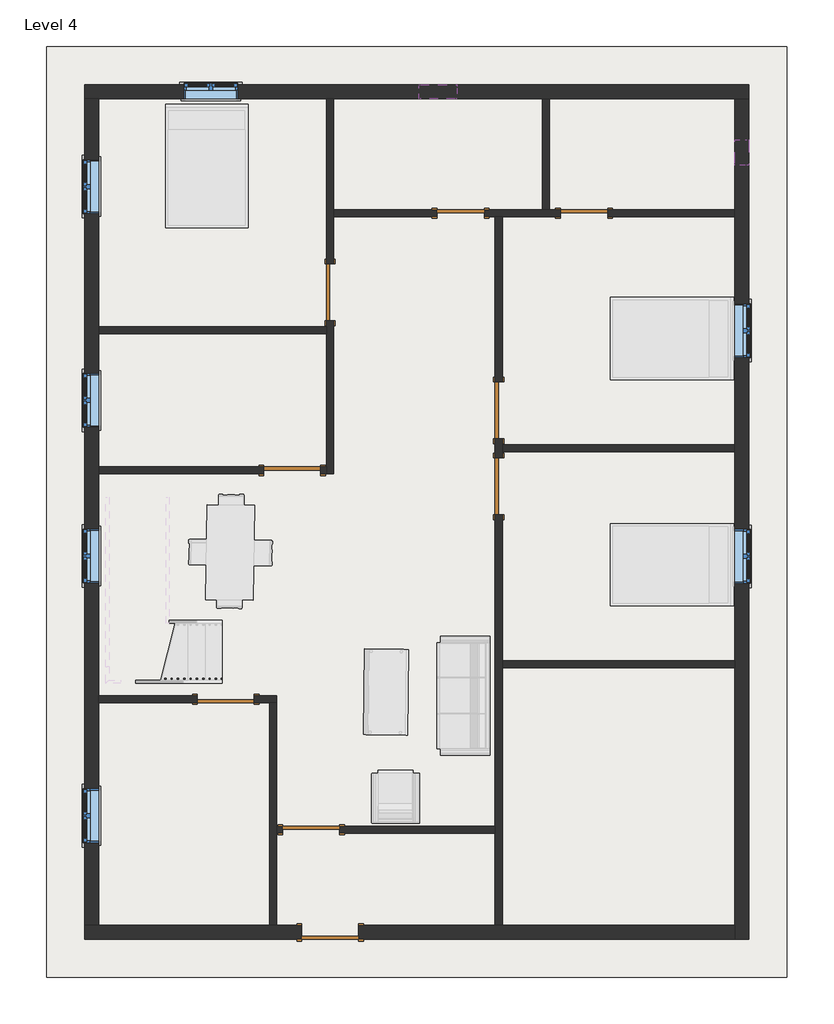
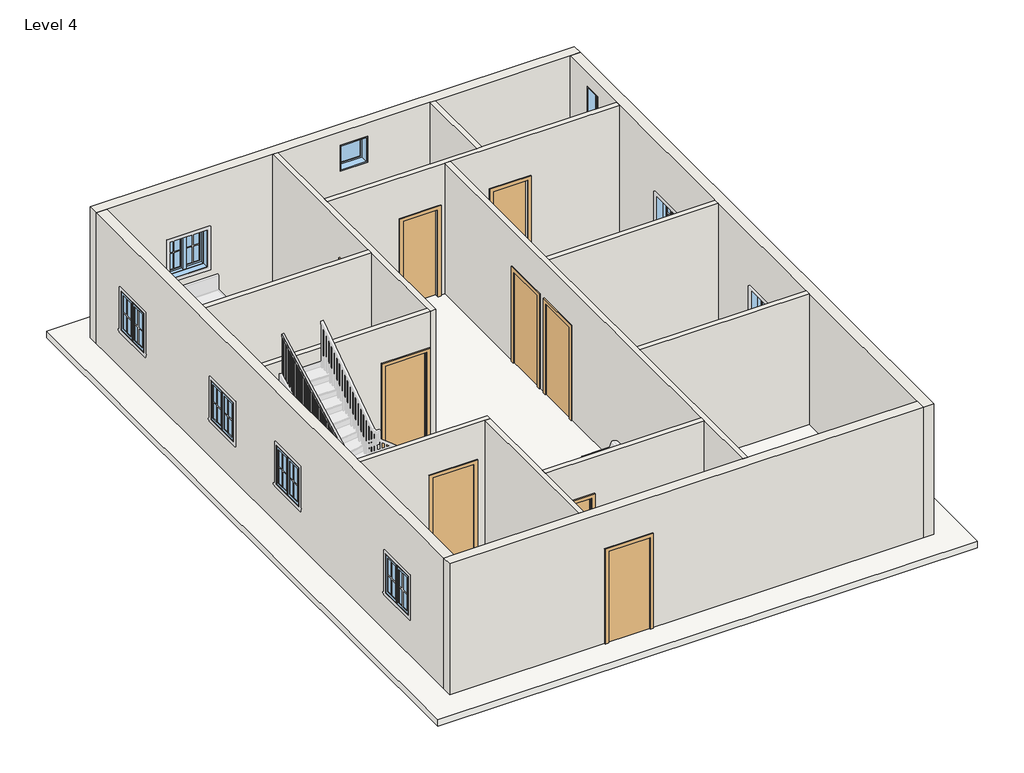
# One storey, part 1 of 2: 15 walls, 9 doors, 9 windows, 1 railing, 1 roof.
"""IFC4 building model written with IfcOpenShell, lengths in millimetres."""

from ifc_helpers import new_model, si_unit, frame, origin, place, context, project, spatial, polyline, outline, extrude, faceted_brep, transform, mapped, element, save
from components import door_d8f5dbb5, door_f2b275c1, door_305aa2a5, door_e5f9f3c4, door_0ca8825f, window_aa618e30, window_80340324, window_339605e1

model = new_model("IFC4")

# Units and contexts
model_context = context("Model", 3, world=origin())
ifc_project = project(units=[si_unit("LENGTHUNIT", "METRE", prefix="MILLI")], contexts=[model_context])

# Site, building, storey
site = spatial("IfcSite", under=ifc_project)
building = spatial("IfcBuilding", under=site)
storey = spatial("IfcBuildingStorey", under=building, Name="Level 4", Elevation=6400.8)

# Doors
placement = place(None, origin())
door_shape = door_d8f5dbb5(model_context)
element("IfcDoor", 1, ObjectType="Single-Flush : 30\" x 80\"", at=placement, inside=storey, context=model_context, shape_type="MappedRepresentation", body=[
    mapped(door_shape, transform((-551.6099931, 5332.4435985, 6400.8), x_axis=(1.0, 0.0, 0.0), y_axis=(0.0, 1.0, 0.0), z_axis=(0.0, 0.0, 1.0))),
])
door_2_shape = door_f2b275c1(model_context)
element("IfcDoor", 2, ObjectType="Single-Flush : 30\" x 80\"", at=placement, inside=storey, context=model_context, shape_type="MappedRepresentation", body=[
    mapped(door_2_shape, transform((1429.5900069, 5332.4435985, 6400.8), x_axis=(-1.0, 0.0, 0.0), y_axis=(0.0, -1.0, 0.0), z_axis=(0.0, 0.0, 1.0))),
])
door_3_shape = door_305aa2a5(model_context)
element("IfcDoor", 3, ObjectType="Single-Flush : 36\" x 84\"", at=placement, inside=storey, context=model_context, shape_type="MappedRepresentation", body=[
    mapped(door_3_shape, transform((-2647.1099931, 4062.4435985, 6400.8), x_axis=(0.0, -1.0, 0.0), y_axis=(1.0, 0.0, 0.0), z_axis=(0.0, 0.0, 1.0))),
])
element("IfcDoor", 4, ObjectType="Single-Flush : 36\" x 84\"", at=placement, inside=storey, context=model_context, shape_type="MappedRepresentation", body=[
    mapped(door_3_shape, transform((57.9900069, 2170.1435985, 6400.8), x_axis=(0.0, -1.0, 0.0), y_axis=(1.0, 0.0, 0.0), z_axis=(0.0, 0.0, 1.0))),
])
element("IfcDoor", 5, ObjectType="Single-Flush : 36\" x 84\"", at=placement, inside=storey, context=model_context, shape_type="MappedRepresentation", body=[
    mapped(door_3_shape, transform((-4323.5099931, -2465.3564015, 6400.8), x_axis=(1.0, 0.0, 0.0), y_axis=(0.0, 1.0, 0.0), z_axis=(0.0, 0.0, 1.0))),
])
element("IfcDoor", 6, ObjectType="Single-Flush : 36\" x 84\"", at=placement, inside=storey, context=model_context, shape_type="MappedRepresentation", body=[
    mapped(door_3_shape, transform((-2951.9099931, -4560.8564015, 6400.8), x_axis=(-1.0, 0.0, 0.0), y_axis=(0.0, -1.0, 0.0), z_axis=(0.0, 0.0, 1.0))),
])
door_4_shape = door_e5f9f3c4(model_context)
element("IfcDoor", 7, ObjectType="Single-Flush : 36\" x 84\"", at=placement, inside=storey, context=model_context, shape_type="MappedRepresentation", body=[
    mapped(door_4_shape, transform((-3256.7099931, 1204.9435985, 6400.8), x_axis=(1.0, 0.0, 0.0), y_axis=(0.0, 1.0, 0.0), z_axis=(0.0, 0.0, 1.0))),
])
element("IfcDoor", 8, ObjectType="Single-Flush : 36\" x 84\"", at=placement, inside=storey, context=model_context, shape_type="MappedRepresentation", body=[
    mapped(door_4_shape, transform((57.9900069, 950.9435985, 6400.8), x_axis=(0.0, 1.0, 0.0), y_axis=(-1.0, 0.0, 0.0), z_axis=(0.0, 0.0, 1.0))),
])
door_5_shape = door_0ca8825f(model_context)
element("IfcDoor", 9, ObjectType="Single-Flush : 36\" x 84\"", at=placement, inside=storey, context=model_context, shape_type="MappedRepresentation", body=[
    mapped(door_5_shape, transform((-2647.1099931, -6205.5064015, 6400.8), x_axis=(-1.0, 0.0, 0.0), y_axis=(0.0, -1.0, 0.0), z_axis=(0.0, 0.0, 1.0))),
])

# Railing
element("IfcRailing", 10, ObjectType="Handrail - Rectangular", at=placement, inside=storey, context=model_context, shape_type="SolidModel", body=[
    faceted_brep([(-4378.4230036, -2160.5564015, 8161.8666667), (-4378.4230036, -2160.5564015, 8105.7107192), (-4378.4230036, -2109.7564015, 8105.7107192), (-4378.4230036, -2109.7564015, 8161.8666667), (-5973.5005957, -2160.5564015, 8913.3835228), (-5984.8684735, -2160.5564015, 8862.5835228), (-5984.8684735, -2109.7564015, 8862.5835228), (-5973.5005957, -2109.7564015, 8913.3835228), (-6196.7599931, -2160.5564015, 8913.3835228), (-6196.7599931, -2160.5564015, 8862.5835228), (-6145.9599931, -2109.7564015, 8862.5835228), (-6145.9599931, -2109.7564015, 8913.3835228), (-6196.7599931, -1959.3194067, 8913.3835228), (-6196.7599931, -1946.6862419, 8862.5835228), (-6145.9599931, -1946.6862419, 8862.5835228), (-6145.9599931, -1959.3194067, 8913.3835228), (-6196.7599931, 775.380588, 10363.2), (-6145.9599931, 775.380588, 10363.2), (-6145.9599931, 775.380588, 10305.7024571), (-6196.7599931, 775.380588, 10305.7024571)], [[[0, 1, 2, 3]], [[1, 0, 4, 5]], [[2, 1, 5, 6]], [[3, 2, 6, 7]], [[0, 3, 7, 4]], [[5, 4, 8, 9]], [[6, 5, 9, 10]], [[7, 6, 10, 11]], [[4, 7, 11, 8]], [[9, 8, 12, 13]], [[10, 9, 13, 14]], [[11, 10, 14, 15]], [[8, 11, 15, 12]], [[16, 17, 18, 19]], [[13, 12, 16, 19]], [[14, 13, 19, 18]], [[15, 14, 18, 17]], [[12, 15, 17, 16]]]),
    extrude(outline(polyline([(719.1685985, 10275.9013569), (719.1685985, 9279.4666667), (700.1185985, 9279.4666667), (700.1185985, 10265.801893), (719.1685985, 10275.9013569)])), frame((-6180.8849931, 0.0, 0.0), z_axis=(1.0, 0.0, 0.0), x_axis=(0.0, 1.0, 0.0)), (0.0, 0.0, 1.0), 19.05),
    extrude(outline(polyline([(617.5685985, 10222.0375494), (617.5685985, 9279.4666667), (598.5185985, 9279.4666667), (598.5185985, 10211.9380855), (617.5685985, 10222.0375494)])), frame((-6180.8849931, 0.0, 0.0), z_axis=(1.0, 0.0, 0.0), x_axis=(0.0, 1.0, 0.0)), (0.0, 0.0, 1.0), 19.05),
    extrude(outline(polyline([(515.9685985, 10168.1737419), (515.9685985, 9279.4666667), (496.9185985, 9279.4666667), (496.9185985, 10158.074278), (515.9685985, 10168.1737419)])), frame((-6180.8849931, 0.0, 0.0), z_axis=(1.0, 0.0, 0.0), x_axis=(0.0, 1.0, 0.0)), (0.0, 0.0, 1.0), 19.05),
    extrude(outline(polyline([(414.3685985, 10114.3099344), (414.3685985, 9110.1333333), (395.3185985, 9110.1333333), (395.3185985, 10104.2104705), (414.3685985, 10114.3099344)])), frame((-6180.8849931, 0.0, 0.0), z_axis=(1.0, 0.0, 0.0), x_axis=(0.0, 1.0, 0.0)), (0.0, 0.0, 1.0), 19.05),
    extrude(outline(polyline([(312.7685985, 10060.4461269), (312.7685985, 9110.1333333), (293.7185985, 9110.1333333), (293.7185985, 10050.346663), (312.7685985, 10060.4461269)])), frame((-6180.8849931, 0.0, 0.0), z_axis=(1.0, 0.0, 0.0), x_axis=(0.0, 1.0, 0.0)), (0.0, 0.0, 1.0), 19.05),
    extrude(outline(polyline([(211.1685985, 10006.5823194), (211.1685985, 8940.8), (192.1185985, 8940.8), (192.1185985, 9996.4828555), (211.1685985, 10006.5823194)])), frame((-6180.8849931, 0.0, 0.0), z_axis=(1.0, 0.0, 0.0), x_axis=(0.0, 1.0, 0.0)), (0.0, 0.0, 1.0), 19.05),
    extrude(outline(polyline([(109.5685985, 9952.7185119), (109.5685985, 8940.8), (90.5185985, 8940.8), (90.5185985, 9942.619048), (109.5685985, 9952.7185119)])), frame((-6180.8849931, 0.0, 0.0), z_axis=(1.0, 0.0, 0.0), x_axis=(0.0, 1.0, 0.0)), (0.0, 0.0, 1.0), 19.05),
    extrude(outline(polyline([(7.9685985, 9898.8547044), (7.9685985, 8940.8), (-11.0814015, 8940.8), (-11.0814015, 9888.7552405), (7.9685985, 9898.8547044)])), frame((-6180.8849931, 0.0, 0.0), z_axis=(1.0, 0.0, 0.0), x_axis=(0.0, 1.0, 0.0)), (0.0, 0.0, 1.0), 19.05),
    extrude(outline(polyline([(-93.6314015, 9844.9908969), (-93.6314015, 8771.4666667), (-112.6814015, 8771.4666667), (-112.6814015, 9834.891433), (-93.6314015, 9844.9908969)])), frame((-6180.8849931, 0.0, 0.0), z_axis=(1.0, 0.0, 0.0), x_axis=(0.0, 1.0, 0.0)), (0.0, 0.0, 1.0), 19.05),
    extrude(outline(polyline([(-195.2314015, 9791.1270894), (-195.2314015, 8771.4666667), (-214.2814015, 8771.4666667), (-214.2814015, 9781.0276255), (-195.2314015, 9791.1270894)])), frame((-6180.8849931, 0.0, 0.0), z_axis=(1.0, 0.0, 0.0), x_axis=(0.0, 1.0, 0.0)), (0.0, 0.0, 1.0), 19.05),
    extrude(outline(polyline([(-296.8314015, 9737.2632819), (-296.8314015, 8771.4666667), (-315.8814015, 8771.4666667), (-315.8814015, 9727.163818), (-296.8314015, 9737.2632819)])), frame((-6180.8849931, 0.0, 0.0), z_axis=(1.0, 0.0, 0.0), x_axis=(0.0, 1.0, 0.0)), (0.0, 0.0, 1.0), 19.05),
    extrude(outline(polyline([(-398.4314015, 9683.3994744), (-398.4314015, 8602.1333333), (-417.4814015, 8602.1333333), (-417.4814015, 9673.3000105), (-398.4314015, 9683.3994744)])), frame((-6180.8849931, 0.0, 0.0), z_axis=(1.0, 0.0, 0.0), x_axis=(0.0, 1.0, 0.0)), (0.0, 0.0, 1.0), 19.05),
    extrude(outline(polyline([(-500.0314015, 9629.5356669), (-500.0314015, 8602.1333333), (-519.0814015, 8602.1333333), (-519.0814015, 9619.436203), (-500.0314015, 9629.5356669)])), frame((-6180.8849931, 0.0, 0.0), z_axis=(1.0, 0.0, 0.0), x_axis=(0.0, 1.0, 0.0)), (0.0, 0.0, 1.0), 19.05),
    extrude(outline(polyline([(-601.6314015, 9575.6718594), (-601.6314015, 8602.1333333), (-620.6814015, 8602.1333333), (-620.6814015, 9565.5723955), (-601.6314015, 9575.6718594)])), frame((-6180.8849931, 0.0, 0.0), z_axis=(1.0, 0.0, 0.0), x_axis=(0.0, 1.0, 0.0)), (0.0, 0.0, 1.0), 19.05),
    extrude(outline(polyline([(-703.2314015, 9521.8080519), (-703.2314015, 8432.8), (-722.2814015, 8432.8), (-722.2814015, 9511.708588), (-703.2314015, 9521.8080519)])), frame((-6180.8849931, 0.0, 0.0), z_axis=(1.0, 0.0, 0.0), x_axis=(0.0, 1.0, 0.0)), (0.0, 0.0, 1.0), 19.05),
    extrude(outline(polyline([(-804.8314015, 9467.9442444), (-804.8314015, 8432.8), (-823.8814015, 8432.8), (-823.8814015, 9457.8447805), (-804.8314015, 9467.9442444)])), frame((-6180.8849931, 0.0, 0.0), z_axis=(1.0, 0.0, 0.0), x_axis=(0.0, 1.0, 0.0)), (0.0, 0.0, 1.0), 19.05),
    extrude(outline(polyline([(-906.4314015, 9414.0804369), (-906.4314015, 8432.8), (-925.4814015, 8432.8), (-925.4814015, 9403.980973), (-906.4314015, 9414.0804369)])), frame((-6180.8849931, 0.0, 0.0), z_axis=(1.0, 0.0, 0.0), x_axis=(0.0, 1.0, 0.0)), (0.0, 0.0, 1.0), 19.05),
    extrude(outline(polyline([(-1008.0314015, 9360.2166294), (-1008.0314015, 8263.4666667), (-1027.0814015, 8263.4666667), (-1027.0814015, 9350.1171655), (-1008.0314015, 9360.2166294)])), frame((-6180.8849931, 0.0, 0.0), z_axis=(1.0, 0.0, 0.0), x_axis=(0.0, 1.0, 0.0)), (0.0, 0.0, 1.0), 19.05),
    extrude(outline(polyline([(-1109.6314015, 9306.3528219), (-1109.6314015, 8263.4666667), (-1128.6814015, 8263.4666667), (-1128.6814015, 9296.253358), (-1109.6314015, 9306.3528219)])), frame((-6180.8849931, 0.0, 0.0), z_axis=(1.0, 0.0, 0.0), x_axis=(0.0, 1.0, 0.0)), (0.0, 0.0, 1.0), 19.05),
    extrude(outline(polyline([(-1211.2314015, 9252.4890144), (-1211.2314015, 8263.4666667), (-1230.2814015, 8263.4666667), (-1230.2814015, 9242.3895505), (-1211.2314015, 9252.4890144)])), frame((-6180.8849931, 0.0, 0.0), z_axis=(1.0, 0.0, 0.0), x_axis=(0.0, 1.0, 0.0)), (0.0, 0.0, 1.0), 19.05),
    extrude(outline(polyline([(-1312.8314015, 9198.6252069), (-1312.8314015, 8263.4666667), (-1331.8814015, 8263.4666667), (-1331.8814015, 9188.525743), (-1312.8314015, 9198.6252069)])), frame((-6180.8849931, 0.0, 0.0), z_axis=(1.0, 0.0, 0.0), x_axis=(0.0, 1.0, 0.0)), (0.0, 0.0, 1.0), 19.05),
    extrude(outline(polyline([(-1414.4314015, 9144.7613994), (-1414.4314015, 8094.1333333), (-1433.4814015, 8094.1333333), (-1433.4814015, 9134.6619355), (-1414.4314015, 9144.7613994)])), frame((-6180.8849931, 0.0, 0.0), z_axis=(1.0, 0.0, 0.0), x_axis=(0.0, 1.0, 0.0)), (0.0, 0.0, 1.0), 19.05),
    extrude(outline(polyline([(-1516.0314015, 9090.8975919), (-1516.0314015, 8094.1333333), (-1535.0814015, 8094.1333333), (-1535.0814015, 9080.798128), (-1516.0314015, 9090.8975919)])), frame((-6180.8849931, 0.0, 0.0), z_axis=(1.0, 0.0, 0.0), x_axis=(0.0, 1.0, 0.0)), (0.0, 0.0, 1.0), 19.05),
    extrude(outline(polyline([(-1617.6314015, 9037.0337844), (-1617.6314015, 8094.1333333), (-1636.6814015, 8094.1333333), (-1636.6814015, 9026.9343205), (-1617.6314015, 9037.0337844)])), frame((-6180.8849931, 0.0, 0.0), z_axis=(1.0, 0.0, 0.0), x_axis=(0.0, 1.0, 0.0)), (0.0, 0.0, 1.0), 19.05),
    extrude(outline(polyline([(-1719.2314015, 8983.1699769), (-1719.2314015, 8094.1333333), (-1738.2814015, 8094.1333333), (-1738.2814015, 8973.070513), (-1719.2314015, 8983.1699769)])), frame((-6180.8849931, 0.0, 0.0), z_axis=(1.0, 0.0, 0.0), x_axis=(0.0, 1.0, 0.0)), (0.0, 0.0, 1.0), 19.05),
    extrude(outline(polyline([(-1820.8314015, 8929.3061694), (-1820.8314015, 7924.8), (-1839.8814015, 7924.8), (-1839.8814015, 8919.2067055), (-1820.8314015, 8929.3061694)])), frame((-6180.8849931, 0.0, 0.0), z_axis=(1.0, 0.0, 0.0), x_axis=(0.0, 1.0, 0.0)), (0.0, 0.0, 1.0), 19.05),
    extrude(outline(polyline([(-1922.4314015, 8875.4423619), (-1922.4314015, 7924.8), (-1941.4814015, 7924.8), (-1941.4814015, 8865.342898), (-1922.4314015, 8875.4423619)])), frame((-6180.8849931, 0.0, 0.0), z_axis=(1.0, 0.0, 0.0), x_axis=(0.0, 1.0, 0.0)), (0.0, 0.0, 1.0), 19.05),
    extrude(outline(polyline([(-6180.8849931, -2043.0814015), (-6180.8849931, -2024.0314015), (-6161.8349931, -2024.0314015), (-6161.8349931, -2043.0814015), (-6180.8849931, -2043.0814015)])), frame((0.0, 0.0, 7924.8), z_axis=(0.0, 0.0, 1.0), x_axis=(1.0, 0.0, 0.0)), (0.0, 0.0, 1.0), 937.7835228),
    extrude(outline(polyline([(-6096.0980036, -2144.6814015), (-6115.1480036, -2144.6814015), (-6115.1480036, -2125.6314015), (-6096.0980036, -2125.6314015), (-6096.0980036, -2144.6814015)])), frame((0.0, 0.0, 7924.8), z_axis=(0.0, 0.0, 1.0), x_axis=(1.0, 0.0, 0.0)), (0.0, 0.0, 1.0), 937.7835228),
    extrude(outline(polyline([(-5994.4980036, -2144.6814015), (-6013.5480036, -2144.6814015), (-6013.5480036, -2125.6314015), (-5994.4980036, -2125.6314015), (-5994.4980036, -2144.6814015)])), frame((0.0, 0.0, 7924.8), z_axis=(0.0, 0.0, 1.0), x_axis=(1.0, 0.0, 0.0)), (0.0, 0.0, 1.0), 937.7835228),
    extrude(outline(polyline([(8828.227224, -5911.9480036), (7924.8, -5911.9480036), (7924.8, -5892.8980036), (8819.2518637, -5892.8980036), (8828.227224, -5911.9480036)])), frame((0.0, -2144.6814015, 0.0), z_axis=(0.0, 1.0, 0.0), x_axis=(0.0, 0.0, 1.0)), (0.0, 0.0, 1.0), 19.05),
    extrude(outline(polyline([(8780.3586357, -5810.3480036), (7924.8, -5810.3480036), (7924.8, -5791.2980036), (8771.3832754, -5791.2980036), (8780.3586357, -5810.3480036)])), frame((0.0, -2144.6814015, 0.0), z_axis=(0.0, 1.0, 0.0), x_axis=(0.0, 0.0, 1.0)), (0.0, 0.0, 1.0), 19.05),
    extrude(outline(polyline([(8732.4900474, -5708.7480036), (7755.4666667, -5708.7480036), (7755.4666667, -5689.6980036), (8723.5146871, -5689.6980036), (8732.4900474, -5708.7480036)])), frame((0.0, -2144.6814015, 0.0), z_axis=(0.0, 1.0, 0.0), x_axis=(0.0, 0.0, 1.0)), (0.0, 0.0, 1.0), 19.05),
    extrude(outline(polyline([(8684.6214591, -5607.1480036), (7755.4666667, -5607.1480036), (7755.4666667, -5588.0980036), (8675.6460988, -5588.0980036), (8684.6214591, -5607.1480036)])), frame((0.0, -2144.6814015, 0.0), z_axis=(0.0, 1.0, 0.0), x_axis=(0.0, 0.0, 1.0)), (0.0, 0.0, 1.0), 19.05),
    extrude(outline(polyline([(8636.7528708, -5505.5480036), (7755.4666667, -5505.5480036), (7755.4666667, -5486.4980036), (8627.7775105, -5486.4980036), (8636.7528708, -5505.5480036)])), frame((0.0, -2144.6814015, 0.0), z_axis=(0.0, 1.0, 0.0), x_axis=(0.0, 0.0, 1.0)), (0.0, 0.0, 1.0), 19.05),
    extrude(outline(polyline([(8588.8842825, -5403.9480036), (7755.4666667, -5403.9480036), (7755.4666667, -5384.8980036), (8579.9089222, -5384.8980036), (8588.8842825, -5403.9480036)])), frame((0.0, -2144.6814015, 0.0), z_axis=(0.0, 1.0, 0.0), x_axis=(0.0, 0.0, 1.0)), (0.0, 0.0, 1.0), 19.05),
    extrude(outline(polyline([(8541.0156942, -5302.3480036), (7586.1333333, -5302.3480036), (7586.1333333, -5283.2980036), (8532.0403338, -5283.2980036), (8541.0156942, -5302.3480036)])), frame((0.0, -2144.6814015, 0.0), z_axis=(0.0, 1.0, 0.0), x_axis=(0.0, 0.0, 1.0)), (0.0, 0.0, 1.0), 19.05),
    extrude(outline(polyline([(8493.1471058, -5200.7480036), (7586.1333333, -5200.7480036), (7586.1333333, -5181.6980036), (8484.1717455, -5181.6980036), (8493.1471058, -5200.7480036)])), frame((0.0, -2144.6814015, 0.0), z_axis=(0.0, 1.0, 0.0), x_axis=(0.0, 0.0, 1.0)), (0.0, 0.0, 1.0), 19.05),
    extrude(outline(polyline([(8445.2785175, -5099.1480036), (7586.1333333, -5099.1480036), (7586.1333333, -5080.0980036), (8436.3031572, -5080.0980036), (8445.2785175, -5099.1480036)])), frame((0.0, -2144.6814015, 0.0), z_axis=(0.0, 1.0, 0.0), x_axis=(0.0, 0.0, 1.0)), (0.0, 0.0, 1.0), 19.05),
    extrude(outline(polyline([(8397.4099292, -4997.5480036), (7586.1333333, -4997.5480036), (7586.1333333, -4978.4980036), (8388.4345689, -4978.4980036), (8397.4099292, -4997.5480036)])), frame((0.0, -2144.6814015, 0.0), z_axis=(0.0, 1.0, 0.0), x_axis=(0.0, 0.0, 1.0)), (0.0, 0.0, 1.0), 19.05),
    extrude(outline(polyline([(8349.5413409, -4895.9480036), (7416.8, -4895.9480036), (7416.8, -4876.8980036), (8340.5659806, -4876.8980036), (8349.5413409, -4895.9480036)])), frame((0.0, -2144.6814015, 0.0), z_axis=(0.0, 1.0, 0.0), x_axis=(0.0, 0.0, 1.0)), (0.0, 0.0, 1.0), 19.05),
    extrude(outline(polyline([(8301.6727526, -4794.3480036), (7416.8, -4794.3480036), (7416.8, -4775.2980036), (8292.6973923, -4775.2980036), (8301.6727526, -4794.3480036)])), frame((0.0, -2144.6814015, 0.0), z_axis=(0.0, 1.0, 0.0), x_axis=(0.0, 0.0, 1.0)), (0.0, 0.0, 1.0), 19.05),
    extrude(outline(polyline([(8253.8041643, -4692.7480036), (7416.8, -4692.7480036), (7416.8, -4673.6980036), (8244.828804, -4673.6980036), (8253.8041643, -4692.7480036)])), frame((0.0, -2144.6814015, 0.0), z_axis=(0.0, 1.0, 0.0), x_axis=(0.0, 0.0, 1.0)), (0.0, 0.0, 1.0), 19.05),
    extrude(outline(polyline([(8205.935576, -4591.1480036), (7247.4666667, -4591.1480036), (7247.4666667, -4572.0980036), (8196.9602157, -4572.0980036), (8205.935576, -4591.1480036)])), frame((0.0, -2144.6814015, 0.0), z_axis=(0.0, 1.0, 0.0), x_axis=(0.0, 0.0, 1.0)), (0.0, 0.0, 1.0), 19.05),
    extrude(outline(polyline([(8158.0669877, -4489.5480036), (7247.4666667, -4489.5480036), (7247.4666667, -4470.4980036), (8149.0916273, -4470.4980036), (8158.0669877, -4489.5480036)])), frame((0.0, -2144.6814015, 0.0), z_axis=(0.0, 1.0, 0.0), x_axis=(0.0, 0.0, 1.0)), (0.0, 0.0, 1.0), 19.05),
    extrude(outline(polyline([(-6161.8349931, -2144.6814015), (-6180.8849931, -2144.6814015), (-6180.8849931, -2125.6314015), (-6161.8349931, -2125.6314015), (-6161.8349931, -2144.6814015)])), frame((0.0, 0.0, 7924.8), z_axis=(0.0, 0.0, 1.0), x_axis=(1.0, 0.0, 0.0)), (0.0, 0.0, 1.0), 937.7835228),
    extrude(outline(polyline([(775.380588, 10305.7024571), (775.380588, 9279.4666667), (756.330588, 9279.4666667), (756.330588, 10295.6029932), (775.380588, 10305.7024571)])), frame((-6180.8849931, 0.0, 0.0), z_axis=(1.0, 0.0, 0.0), x_axis=(0.0, 1.0, 0.0)), (0.0, 0.0, 1.0), 19.05),
    extrude(outline(polyline([(8114.6860795, -4397.4730036), (7247.4666667, -4397.4730036), (7247.4666667, -4378.4230036), (8105.7107192, -4378.4230036), (8114.6860795, -4397.4730036)])), frame((0.0, -2144.6814015, 0.0), z_axis=(0.0, 1.0, 0.0), x_axis=(0.0, 0.0, 1.0)), (0.0, 0.0, 1.0), 19.05),
])

# Roof
element("IfcRoof", 11, ObjectType="Generic - 12\"", at=placement, inside=storey, context=model_context, shape_type="SweptSolid", body=[
    extrude(outline(polyline([(-7200.0599931, 8005.7935985), (4687.1400069, 8005.7935985), (4687.1400069, -6929.4064015), (-7200.0599931, -6929.4064015), (-7200.0599931, 8005.7935985)])), frame((0.0, 0.0, 6248.4), z_axis=(0.0, 0.0, 1.0), x_axis=(1.0, 0.0, 0.0)), (0.0, 0.0, 1.0), 152.4),
])

# Walls
element("IfcWall", 12, ObjectType="WALL4.5\"", at=placement, inside=storey, context=model_context, shape_type="SweptSolid", body=[
    extrude(outline(polyline([(-2704.2599931, 3395.6935985), (-6361.8599931, 3395.6935985), (-6361.8599931, 3509.9935985), (-2704.2599931, 3509.9935985), (-2704.2599931, 3395.6935985)])), frame((0.0, 0.0, 6400.8), z_axis=(0.0, 0.0, 1.0), x_axis=(1.0, 0.0, 0.0)), (0.0, 0.0, 1.0), 3048.0),
])
element("IfcWall", 13, ObjectType="WALL4.5\"", at=placement, inside=storey, context=model_context, shape_type="Brep", body=[
    faceted_brep([(-2704.2599931, 3605.2435985, 8534.4), (-2704.2599931, 3605.2435985, 6400.8), (-2704.2599931, 3509.9935985, 6400.8), (-2704.2599931, 3395.6935985, 6400.8), (-2704.2599931, 1262.0935985, 6400.8), (-2704.2599931, 1147.7935985, 6400.8), (-2704.2599931, 1147.7935985, 9448.8), (-2704.2599931, 1262.0935985, 9448.8), (-2704.2599931, 3395.6935985, 9448.8), (-2704.2599931, 3509.9935985, 9448.8), (-2704.2599931, 7167.5935985, 9448.8), (-2704.2599931, 7167.5935985, 6400.8), (-2704.2599931, 4519.6435985, 6400.8), (-2704.2599931, 4519.6435985, 8534.4), (-2589.9599931, 1147.7935985, 6400.8), (-2589.9599931, 3605.2435985, 6400.8), (-2589.9599931, 3605.2435985, 8534.4), (-2589.9599931, 4519.6435985, 8534.4), (-2589.9599931, 4519.6435985, 6400.8), (-2589.9599931, 5275.2935985, 6400.8), (-2589.9599931, 5389.5935985, 6400.8), (-2589.9599931, 7167.5935985, 6400.8), (-2589.9599931, 7167.5935985, 9448.8), (-2589.9599931, 5389.5935985, 9448.8), (-2589.9599931, 5275.2935985, 9448.8), (-2589.9599931, 1147.7935985, 9448.8)], [[[0, 1, 2, 3, 4, 5, 6, 7, 8, 9, 10, 11, 12, 13]], [[14, 15, 16, 17, 18, 19, 20, 21, 22, 23, 24, 25]], [[12, 11, 21, 20, 19, 18]], [[5, 4, 3, 2, 1, 15, 14]], [[11, 10, 22, 21]], [[6, 5, 14, 25]], [[16, 15, 1, 0]], [[17, 16, 0, 13]], [[18, 17, 13, 12]], [[10, 9, 8, 7, 6, 25, 24, 23, 22]]]),
])
element("IfcWall", 14, ObjectType="WALL4.5\"", at=placement, inside=storey, context=model_context, shape_type="SweptSolid", body=[
    extrude(outline(polyline([(8534.4, -2799.5099931), (6400.8, -2799.5099931), (6400.8, -2704.2599931), (9448.8, -2704.2599931), (9448.8, -6361.8599931), (6400.8, -6361.8599931), (6400.8, -3713.9099931), (8534.4, -3713.9099931), (8534.4, -2799.5099931)])), frame((0.0, 1147.7935985, 0.0), z_axis=(0.0, 1.0, 0.0), x_axis=(0.0, 0.0, 1.0)), (0.0, 0.0, 1.0), 114.3),
])
element("IfcWall", 15, ObjectType="WALL4.5\"", at=placement, inside=storey, context=model_context, shape_type="Brep", body=[
    faceted_brep([(-170.6099931, 5275.2935985, 6400.8), (0.8400069, 5275.2935985, 6400.8), (115.1400069, 5275.2935985, 6400.8), (1048.5900069, 5275.2935985, 6400.8), (1048.5900069, 5275.2935985, 8432.8), (1810.5900069, 5275.2935985, 8432.8), (1810.5900069, 5275.2935985, 6400.8), (3848.9400069, 5275.2935985, 6400.8), (3848.9400069, 5275.2935985, 9448.8), (115.1400069, 5275.2935985, 9448.8), (0.8400069, 5275.2935985, 9448.8), (-2589.9599931, 5275.2935985, 9448.8), (-2589.9599931, 5275.2935985, 6400.8), (-932.6099931, 5275.2935985, 6400.8), (-932.6099931, 5275.2935985, 8432.8), (-170.6099931, 5275.2935985, 8432.8), (1048.5900069, 5389.5935985, 8432.8), (1048.5900069, 5389.5935985, 6400.8), (877.1400069, 5389.5935985, 6400.8), (762.8400069, 5389.5935985, 6400.8), (-170.6099931, 5389.5935985, 6400.8), (-170.6099931, 5389.5935985, 8432.8), (-932.6099931, 5389.5935985, 8432.8), (-932.6099931, 5389.5935985, 6400.8), (-2589.9599931, 5389.5935985, 6400.8), (-2589.9599931, 5389.5935985, 9448.8), (762.8400069, 5389.5935985, 9448.8), (877.1400069, 5389.5935985, 9448.8), (3848.9400069, 5389.5935985, 9448.8), (3848.9400069, 5389.5935985, 6400.8), (1810.5900069, 5389.5935985, 6400.8), (1810.5900069, 5389.5935985, 8432.8)], [[[0, 1, 2, 3, 4, 5, 6, 7, 8, 9, 10, 11, 12, 13, 14, 15]], [[16, 17, 18, 19, 20, 21, 22, 23, 24, 25, 26, 27, 28, 29, 30, 31]], [[13, 12, 24, 23]], [[30, 29, 7, 6]], [[20, 19, 18, 17, 3, 2, 1, 0]], [[8, 7, 29, 28]], [[12, 11, 25, 24]], [[21, 20, 0, 15]], [[22, 21, 15, 14]], [[23, 22, 14, 13]], [[4, 3, 17, 16]], [[5, 4, 16, 31]], [[6, 5, 31, 30]], [[11, 10, 9, 8, 28, 27, 26, 25]]]),
])
element("IfcWall", 16, ObjectType="WALL4.5\"", at=placement, inside=storey, context=model_context, shape_type="SweptSolid", body=[
    extrude(outline(polyline([(762.8400069, 5389.5935985), (762.8400069, 7167.5935985), (877.1400069, 7167.5935985), (877.1400069, 5389.5935985), (762.8400069, 5389.5935985)])), frame((0.0, 0.0, 6400.8), z_axis=(0.0, 0.0, 1.0), x_axis=(1.0, 0.0, 0.0)), (0.0, 0.0, 1.0), 3048.0),
])
element("IfcWall", 17, ObjectType="WALL4.5\"", at=placement, inside=storey, context=model_context, shape_type="Brep", body=[
    faceted_brep([(0.8400069, 1712.9435985, 6400.8), (0.8400069, 1408.1435985, 6400.8), (0.8400069, 1408.1435985, 8534.4), (0.8400069, 493.7435985, 8534.4), (0.8400069, 493.7435985, 6400.8), (0.8400069, -4503.7064015, 6400.8), (0.8400069, -4618.0064015, 6400.8), (0.8400069, -6091.2064015, 6400.8), (0.8400069, -6091.2064015, 9448.8), (0.8400069, -4618.0064015, 9448.8), (0.8400069, -4503.7064015, 9448.8), (0.8400069, 5275.2935985, 9448.8), (0.8400069, 5275.2935985, 6400.8), (0.8400069, 2627.3435985, 6400.8), (0.8400069, 2627.3435985, 8534.4), (0.8400069, 1712.9435985, 8534.4), (115.1400069, 1408.1435985, 8534.4), (115.1400069, 1408.1435985, 6400.8), (115.1400069, 1503.3935985, 6400.8), (115.1400069, 1617.6935985, 6400.8), (115.1400069, 1712.9435985, 6400.8), (115.1400069, 1712.9435985, 8534.4), (115.1400069, 2627.3435985, 8534.4), (115.1400069, 2627.3435985, 6400.8), (115.1400069, 5275.2935985, 6400.8), (115.1400069, 5275.2935985, 9448.8), (115.1400069, 1617.6935985, 9448.8), (115.1400069, 1503.3935985, 9448.8), (115.1400069, -1850.058017, 9448.8), (115.1400069, -1964.358017, 9448.8), (115.1400069, -6091.2064015, 9448.8), (115.1400069, -6091.2064015, 6400.8), (115.1400069, -1964.358017, 6400.8), (115.1400069, -1850.058017, 6400.8), (115.1400069, 493.7435985, 6400.8), (115.1400069, 493.7435985, 8534.4)], [[[0, 1, 2, 3, 4, 5, 6, 7, 8, 9, 10, 11, 12, 13, 14, 15]], [[16, 17, 18, 19, 20, 21, 22, 23, 24, 25, 26, 27, 28, 29, 30, 31, 32, 33, 34, 35]], [[13, 12, 24, 23]], [[34, 33, 32, 31, 7, 6, 5, 4]], [[20, 19, 18, 17, 1, 0]], [[8, 7, 31, 30]], [[12, 11, 25, 24]], [[21, 20, 0, 15]], [[22, 21, 15, 14]], [[23, 22, 14, 13]], [[2, 1, 17, 16]], [[3, 2, 16, 35]], [[4, 3, 35, 34]], [[11, 10, 9, 8, 30, 29, 28, 27, 26, 25]]]),
])
element("IfcWall", 18, ObjectType="WALL4.5\"", at=placement, inside=storey, context=model_context, shape_type="SweptSolid", body=[
    extrude(outline(polyline([(3848.9400069, -1964.358017), (115.1400069, -1964.358017), (115.1400069, -1850.058017), (3848.9400069, -1850.058017), (3848.9400069, -1964.358017)])), frame((0.0, 0.0, 6400.8), z_axis=(0.0, 0.0, 1.0), x_axis=(1.0, 0.0, 0.0)), (0.0, 0.0, 1.0), 3048.0),
])
element("IfcWall", 19, ObjectType="WALL4.5\"", at=placement, inside=storey, context=model_context, shape_type="SweptSolid", body=[
    extrude(outline(polyline([(3848.9400069, 1503.3935985), (115.1400069, 1503.3935985), (115.1400069, 1617.6935985), (3848.9400069, 1617.6935985), (3848.9400069, 1503.3935985)])), frame((0.0, 0.0, 6400.8), z_axis=(0.0, 0.0, 1.0), x_axis=(1.0, 0.0, 0.0)), (0.0, 0.0, 1.0), 3048.0),
])
element("IfcWall", 20, ObjectType="WALL4.5\"", at=placement, inside=storey, context=model_context, shape_type="Brep", body=[
    faceted_brep([(-3866.3099931, -2522.5064015, 8534.4), (-3866.3099931, -2522.5064015, 6400.8), (-3618.6599931, -2522.5064015, 6400.8), (-3504.3599931, -2522.5064015, 6400.8), (-3504.3599931, -2522.5064015, 9448.8), (-3618.6599931, -2522.5064015, 9448.8), (-6361.8599931, -2522.5064015, 9448.8), (-6361.8599931, -2522.5064015, 6400.8), (-4780.7099931, -2522.5064015, 6400.8), (-4780.7099931, -2522.5064015, 8534.4), (-3504.3599931, -2408.2064015, 6400.8), (-3866.3099931, -2408.2064015, 6400.8), (-3866.3099931, -2408.2064015, 8534.4), (-4780.7099931, -2408.2064015, 8534.4), (-4780.7099931, -2408.2064015, 6400.8), (-6361.8599931, -2408.2064015, 6400.8), (-6361.8599931, -2408.2064015, 9448.8), (-3504.3599931, -2408.2064015, 9448.8)], [[[0, 1, 2, 3, 4, 5, 6, 7, 8, 9]], [[10, 11, 12, 13, 14, 15, 16, 17]], [[8, 7, 15, 14]], [[3, 2, 1, 11, 10]], [[7, 6, 16, 15]], [[4, 3, 10, 17]], [[12, 11, 1, 0]], [[13, 12, 0, 9]], [[14, 13, 9, 8]], [[6, 5, 4, 17, 16]]]),
])
element("IfcWall", 21, ObjectType="WALL4.5\"", at=placement, inside=storey, context=model_context, shape_type="SweptSolid", body=[
    extrude(outline(polyline([(6400.8, -3504.3599931), (6400.8, -3409.1099931), (8534.4, -3409.1099931), (8534.4, -2494.7099931), (6400.8, -2494.7099931), (6400.8, 0.8400069), (9448.8, 0.8400069), (9448.8, -3504.3599931), (6400.8, -3504.3599931)])), frame((0.0, -4618.0064015, 0.0), z_axis=(0.0, 1.0, 0.0), x_axis=(0.0, 0.0, 1.0)), (0.0, 0.0, 1.0), 114.3),
])
element("IfcWall", 22, ObjectType="WALL4.5\"", at=placement, inside=storey, context=model_context, shape_type="Brep", body=[
    faceted_brep([(-3504.3599931, -6091.2064015, 6400.8), (-3504.3599931, -4618.0064015, 6400.8), (-3504.3599931, -4503.7064015, 6400.8), (-3504.3599931, -2522.5064015, 6400.8), (-3504.3599931, -2522.5064015, 9448.8), (-3504.3599931, -4503.7064015, 9448.8), (-3504.3599931, -4618.0064015, 9448.8), (-3504.3599931, -6091.2064015, 9448.8), (-3618.6599931, -6091.2064015, 6400.8), (-3618.6599931, -6091.2064015, 9448.8), (-3618.6599931, -2522.5064015, 9448.8), (-3618.6599931, -2522.5064015, 6400.8)], [[[0, 1, 2, 3, 4, 5, 6, 7]], [[8, 9, 10, 11]], [[3, 2, 1, 0, 8, 11]], [[4, 3, 11, 10]], [[0, 7, 9, 8]], [[7, 6, 5, 4, 10, 9]]]),
])
element("IfcWall", 23, ObjectType="WALL9\"", at=placement, inside=storey, context=model_context, shape_type="Brep", body=[
    faceted_brep([(-6590.4599931, 7167.5935985, 6400.8), (-6361.8599931, 7167.5935985, 6400.8), (-2704.2599931, 7167.5935985, 6400.8), (-2589.9599931, 7167.5935985, 6400.8), (762.8400069, 7167.5935985, 6400.8), (877.1400069, 7167.5935985, 6400.8), (3848.9400069, 7167.5935985, 6400.8), (4077.5400069, 7167.5935985, 6400.8), (4077.5400069, 7167.5935985, 9448.8), (3848.9400069, 7167.5935985, 9448.8), (877.1400069, 7167.5935985, 9448.8), (762.8400069, 7167.5935985, 9448.8), (-2589.9599931, 7167.5935985, 9448.8), (-2704.2599931, 7167.5935985, 9448.8), (-6361.8599931, 7167.5935985, 9448.8), (-6590.4599931, 7167.5935985, 9448.8), (-608.7599931, 7167.5935985, 9144.0), (-608.7599931, 7167.5935985, 8534.4), (-1218.3599931, 7167.5935985, 8534.4), (-1218.3599931, 7167.5935985, 9144.0), (-4129.8349931, 7167.5935985, 8229.6), (-4129.8349931, 7167.5935985, 7315.2), (-4993.4349931, 7167.5935985, 7315.2), (-4993.4349931, 7167.5935985, 8229.6), (4077.5400069, 7396.1935985, 6400.8), (-6590.4599931, 7396.1935985, 6400.8), (-6590.4599931, 7396.1935985, 9448.8), (4077.5400069, 7396.1935985, 9448.8), (-608.7599931, 7396.1935985, 8534.4), (-608.7599931, 7396.1935985, 9144.0), (-1218.3599931, 7396.1935985, 9144.0), (-1218.3599931, 7396.1935985, 8534.4), (-4129.8349931, 7396.1935985, 7315.2), (-4129.8349931, 7396.1935985, 8229.6), (-4993.4349931, 7396.1935985, 8229.6), (-4993.4349931, 7396.1935985, 7315.2)], [[[0, 1, 2, 3, 4, 5, 6, 7, 8, 9, 10, 11, 12, 13, 14, 15], [16, 17, 18, 19], [20, 21, 22, 23]], [[24, 25, 26, 27], [28, 29, 30, 31], [32, 33, 34, 35]], [[7, 6, 5, 4, 3, 2, 1, 0, 25, 24]], [[8, 7, 24, 27]], [[0, 15, 26, 25]], [[16, 29, 28, 17]], [[17, 28, 31, 18]], [[18, 31, 30, 19]], [[21, 20, 33, 32]], [[22, 21, 32, 35]], [[23, 22, 35, 34]], [[20, 23, 34, 33]], [[15, 14, 13, 12, 11, 10, 9, 8, 27, 26]], [[29, 16, 19, 30]]]),
])
element("IfcWall", 24, ObjectType="WALL9\"", at=placement, inside=storey, context=model_context, shape_type="Brep", body=[
    faceted_brep([(3848.9400069, 7167.5935985, 6400.8), (3848.9400069, 5389.5935985, 6400.8), (3848.9400069, 5275.2935985, 6400.8), (3848.9400069, 1617.6935985, 6400.8), (3848.9400069, 1503.3935985, 6400.8), (3848.9400069, -1850.058017, 6400.8), (3848.9400069, -1964.358017, 6400.8), (3848.9400069, -6091.2064015, 6400.8), (3848.9400069, -6319.8064015, 6400.8), (3848.9400069, -6319.8064015, 9448.8), (3848.9400069, -6091.2064015, 9448.8), (3848.9400069, -1964.358017, 9448.8), (3848.9400069, -1850.058017, 9448.8), (3848.9400069, 1503.3935985, 9448.8), (3848.9400069, 1617.6935985, 9448.8), (3848.9400069, 5275.2935985, 9448.8), (3848.9400069, 5389.5935985, 9448.8), (3848.9400069, 7167.5935985, 9448.8), (3848.9400069, 6103.9685985, 9144.0), (3848.9400069, 6103.9685985, 8534.4), (3848.9400069, 6510.3685985, 8534.4), (3848.9400069, 6510.3685985, 9144.0), (3848.9400069, 3014.6935985, 8229.6), (3848.9400069, 3014.6935985, 7315.2), (3848.9400069, 3878.2935985, 7315.2), (3848.9400069, 3878.2935985, 8229.6), (3848.9400069, -605.1322092, 8229.6), (3848.9400069, -605.1322092, 7315.2), (3848.9400069, 258.4677908, 7315.2), (3848.9400069, 258.4677908, 8229.6), (4077.5400069, -6319.8064015, 6400.8), (4077.5400069, 7167.5935985, 6400.8), (4077.5400069, 7167.5935985, 9448.8), (4077.5400069, -6319.8064015, 9448.8), (4077.5400069, 6103.9685985, 8534.4), (4077.5400069, 6103.9685985, 9144.0), (4077.5400069, 6510.3685985, 9144.0), (4077.5400069, 6510.3685985, 8534.4), (4077.5400069, 3014.6935985, 7315.2), (4077.5400069, 3014.6935985, 8229.6), (4077.5400069, 3878.2935985, 8229.6), (4077.5400069, 3878.2935985, 7315.2), (4077.5400069, -605.1322092, 7315.2), (4077.5400069, -605.1322092, 8229.6), (4077.5400069, 258.4677908, 8229.6), (4077.5400069, 258.4677908, 7315.2)], [[[0, 1, 2, 3, 4, 5, 6, 7, 8, 9, 10, 11, 12, 13, 14, 15, 16, 17], [18, 19, 20, 21], [22, 23, 24, 25], [26, 27, 28, 29]], [[30, 31, 32, 33], [34, 35, 36, 37], [38, 39, 40, 41], [42, 43, 44, 45]], [[8, 7, 6, 5, 4, 3, 2, 1, 0, 31, 30]], [[0, 17, 32, 31]], [[9, 8, 30, 33]], [[18, 35, 34, 19]], [[19, 34, 37, 20]], [[20, 37, 36, 21]], [[23, 22, 39, 38]], [[24, 23, 38, 41]], [[25, 24, 41, 40]], [[22, 25, 40, 39]], [[27, 26, 43, 42]], [[28, 27, 42, 45]], [[29, 28, 45, 44]], [[26, 29, 44, 43]], [[17, 16, 15, 14, 13, 12, 11, 10, 9, 33, 32]], [[35, 18, 21, 36]]]),
])
element("IfcWall", 25, ObjectType="WALL9\"", at=placement, inside=storey, context=model_context, shape_type="Brep", body=[
    faceted_brep([(-3104.3099931, -6091.2064015, 8534.4), (-3104.3099931, -6091.2064015, 6400.8), (-3504.3599931, -6091.2064015, 6400.8), (-3618.6599931, -6091.2064015, 6400.8), (-6361.8599931, -6091.2064015, 6400.8), (-6590.4599931, -6091.2064015, 6400.8), (-6590.4599931, -6091.2064015, 9448.8), (-6361.8599931, -6091.2064015, 9448.8), (-3618.6599931, -6091.2064015, 9448.8), (-3504.3599931, -6091.2064015, 9448.8), (0.8400069, -6091.2064015, 9448.8), (115.1400069, -6091.2064015, 9448.8), (3848.9400069, -6091.2064015, 9448.8), (3848.9400069, -6091.2064015, 6400.8), (115.1400069, -6091.2064015, 6400.8), (0.8400069, -6091.2064015, 6400.8), (-2189.9099931, -6091.2064015, 6400.8), (-2189.9099931, -6091.2064015, 8534.4), (-6590.4599931, -6319.8064015, 6400.8), (-3104.3099931, -6319.8064015, 6400.8), (-3104.3099931, -6319.8064015, 8534.4), (-2189.9099931, -6319.8064015, 8534.4), (-2189.9099931, -6319.8064015, 6400.8), (3848.9400069, -6319.8064015, 6400.8), (3848.9400069, -6319.8064015, 9448.8), (-6590.4599931, -6319.8064015, 9448.8)], [[[0, 1, 2, 3, 4, 5, 6, 7, 8, 9, 10, 11, 12, 13, 14, 15, 16, 17]], [[18, 19, 20, 21, 22, 23, 24, 25]], [[5, 4, 3, 2, 1, 19, 18]], [[16, 15, 14, 13, 23, 22]], [[13, 12, 24, 23]], [[6, 5, 18, 25]], [[12, 11, 10, 9, 8, 7, 6, 25, 24]], [[20, 19, 1, 0]], [[21, 20, 0, 17]], [[22, 21, 17, 16]]]),
])
element("IfcWall", 26, ObjectType="WALL9\"", at=placement, inside=storey, context=model_context, shape_type="Brep", body=[
    faceted_brep([(-6361.8599931, -6091.2064015, 6400.8), (-6361.8599931, -2522.5064015, 6400.8), (-6361.8599931, -2408.2064015, 6400.8), (-6361.8599931, 1147.7935985, 6400.8), (-6361.8599931, 1262.0935985, 6400.8), (-6361.8599931, 3395.6935985, 6400.8), (-6361.8599931, 3509.9935985, 6400.8), (-6361.8599931, 7167.5935985, 6400.8), (-6361.8599931, 7167.5935985, 9448.8), (-6361.8599931, 3509.9935985, 9448.8), (-6361.8599931, 3395.6935985, 9448.8), (-6361.8599931, 1262.0935985, 9448.8), (-6361.8599931, 1147.7935985, 9448.8), (-6361.8599931, -2408.2064015, 9448.8), (-6361.8599931, -2522.5064015, 9448.8), (-6361.8599931, -6091.2064015, 9448.8), (-6361.8599931, 2760.6935985, 8229.6), (-6361.8599931, 2760.6935985, 7315.2), (-6361.8599931, 1897.0935985, 7315.2), (-6361.8599931, 1897.0935985, 8229.6), (-6361.8599931, 6189.6935985, 8229.6), (-6361.8599931, 6189.6935985, 7315.2), (-6361.8599931, 5326.0935985, 7315.2), (-6361.8599931, 5326.0935985, 8229.6), (-6361.8599931, -3903.6314015, 8229.6), (-6361.8599931, -3903.6314015, 7315.2), (-6361.8599931, -4767.2314015, 7315.2), (-6361.8599931, -4767.2314015, 8229.6), (-6361.8599931, 265.1435985, 8229.6), (-6361.8599931, 265.1435985, 7315.2), (-6361.8599931, -598.4564015, 7315.2), (-6361.8599931, -598.4564015, 8229.6), (-6590.4599931, -6091.2064015, 6400.8), (-6590.4599931, -6091.2064015, 9448.8), (-6590.4599931, 7167.5935985, 9448.8), (-6590.4599931, 7167.5935985, 6400.8), (-6590.4599931, 2760.6935985, 8229.6), (-6590.4599931, 1897.0935985, 8229.6), (-6590.4599931, 1897.0935985, 7315.2), (-6590.4599931, 2760.6935985, 7315.2), (-6590.4599931, 6189.6935985, 8229.6), (-6590.4599931, 5326.0935985, 8229.6), (-6590.4599931, 5326.0935985, 7315.2), (-6590.4599931, 6189.6935985, 7315.2), (-6590.4599931, -3903.6314015, 8229.6), (-6590.4599931, -4767.2314015, 8229.6), (-6590.4599931, -4767.2314015, 7315.2), (-6590.4599931, -3903.6314015, 7315.2), (-6590.4599931, 265.1435985, 8229.6), (-6590.4599931, -598.4564015, 8229.6), (-6590.4599931, -598.4564015, 7315.2), (-6590.4599931, 265.1435985, 7315.2)], [[[0, 1, 2, 3, 4, 5, 6, 7, 8, 9, 10, 11, 12, 13, 14, 15], [16, 17, 18, 19], [20, 21, 22, 23], [24, 25, 26, 27], [28, 29, 30, 31]], [[32, 33, 34, 35], [36, 37, 38, 39], [40, 41, 42, 43], [44, 45, 46, 47], [48, 49, 50, 51]], [[7, 6, 5, 4, 3, 2, 1, 0, 32, 35]], [[0, 15, 33, 32]], [[8, 7, 35, 34]], [[17, 16, 36, 39]], [[18, 17, 39, 38]], [[19, 18, 38, 37]], [[16, 19, 37, 36]], [[21, 20, 40, 43]], [[22, 21, 43, 42]], [[23, 22, 42, 41]], [[20, 23, 41, 40]], [[25, 24, 44, 47]], [[26, 25, 47, 46]], [[27, 26, 46, 45]], [[24, 27, 45, 44]], [[29, 28, 48, 51]], [[30, 29, 51, 50]], [[31, 30, 50, 49]], [[28, 31, 49, 48]], [[15, 14, 13, 12, 11, 10, 9, 8, 34, 33]]]),
])

# Windows
window_shape = window_aa618e30(model_context)
element("IfcWindow", 27, ObjectType="Fixed : 16\" x 24\"", at=placement, inside=storey, context=model_context, shape_type="MappedRepresentation", body=[
    mapped(window_shape, transform((3963.2400069, 6269.0685985, 7620.0), x_axis=(0.0, -1.0, 0.0), y_axis=(1.0, 0.0, 0.0), z_axis=(0.0, 0.0, 1.0))),
])
window_2_shape = window_80340324(model_context)
element("IfcWindow", 28, ObjectType="Fixed : 24\" x 24\"", at=placement, inside=storey, context=model_context, shape_type="MappedRepresentation", body=[
    mapped(window_2_shape, transform((-875.4599931, 7281.8935985, 7620.0), x_axis=(1.0, 0.0, 0.0), y_axis=(0.0, 1.0, 0.0), z_axis=(0.0, 0.0, 1.0))),
])
window_3_shape = window_339605e1(model_context)
element("IfcWindow", 29, ObjectType="Window-Casement-Double : 34\" x 36\"", at=placement, inside=storey, context=model_context, shape_type="MappedRepresentation", body=[
    mapped(window_3_shape, transform((-4561.6349931, 7281.8935985, 6400.8), x_axis=(1.0, 0.0, 0.0), y_axis=(0.0, 1.0, 0.0), z_axis=(0.0, 0.0, 1.0))),
])
element("IfcWindow", 30, ObjectType="Window-Casement-Double : 34\" x 36\"", at=placement, inside=storey, context=model_context, shape_type="MappedRepresentation", body=[
    mapped(window_3_shape, transform((3963.2400069, 3446.4935985, 6400.8), x_axis=(0.0, -1.0, 0.0), y_axis=(1.0, 0.0, 0.0), z_axis=(0.0, 0.0, 1.0))),
])
element("IfcWindow", 31, ObjectType="Window-Casement-Double : 34\" x 36\"", at=placement, inside=storey, context=model_context, shape_type="MappedRepresentation", body=[
    mapped(window_3_shape, transform((3963.2400069, -173.3322092, 6400.8), x_axis=(0.0, -1.0, 0.0), y_axis=(1.0, 0.0, 0.0), z_axis=(0.0, 0.0, 1.0))),
])
element("IfcWindow", 32, ObjectType="Window-Casement-Double : 34\" x 36\"", at=placement, inside=storey, context=model_context, shape_type="MappedRepresentation", body=[
    mapped(window_3_shape, transform((-6476.1599931, 2328.8935985, 6400.8), x_axis=(0.0, 1.0, 0.0), y_axis=(-1.0, 0.0, 0.0), z_axis=(0.0, 0.0, 1.0))),
])
element("IfcWindow", 33, ObjectType="Window-Casement-Double : 34\" x 36\"", at=placement, inside=storey, context=model_context, shape_type="MappedRepresentation", body=[
    mapped(window_3_shape, transform((-6476.1599931, 5757.8935985, 6400.8), x_axis=(0.0, 1.0, 0.0), y_axis=(-1.0, 0.0, 0.0), z_axis=(0.0, 0.0, 1.0))),
])
element("IfcWindow", 34, ObjectType="Window-Casement-Double : 34\" x 36\"", at=placement, inside=storey, context=model_context, shape_type="MappedRepresentation", body=[
    mapped(window_3_shape, transform((-6476.1599931, -4335.4314015, 6400.8), x_axis=(0.0, 1.0, 0.0), y_axis=(-1.0, 0.0, 0.0), z_axis=(0.0, 0.0, 1.0))),
])
element("IfcWindow", 35, ObjectType="Window-Casement-Double : 34\" x 36\"", at=placement, inside=storey, context=model_context, shape_type="MappedRepresentation", body=[
    mapped(window_3_shape, transform((-6476.1599931, -166.6564015, 6400.8), x_axis=(0.0, 1.0, 0.0), y_axis=(-1.0, 0.0, 0.0), z_axis=(0.0, 0.0, 1.0))),
])

save(model, "model.ifc")

# Revit data of these elements
# Type "Single-Flush : 30\" x 80\""
#   Type Mark = "5"
#   Construction Type Id = "MDOOR"
#   Assembly Code = "C1020"
#   Analytic Construction = "Metal"
#   Thickness = 0' - 2"
#   Heat Transfer Coefficient (U) = 0.651978 BTU/(h·ft²·°F)
#   Height = 6' - 8"
#   Trim Projection Ext = 0' - 1"
#   Trim Projection Int = 0' - 1"
#   Trim Width = 0' - 3"
#   Width = 2' - 6"
#   Define Thermal Properties by = 1
#   Define Thermal Properties by = 1
#   Door Material = Door - Panel
#   Frame Material = Door - Frame
#   Visual Light Transmittance = 0
#   Solar Heat Gain Coefficient = 0
#   Function = (empty or 0)
#   Wall Closure = (empty or 0)
# Type "Single-Flush : 36\" x 84\""
#   Type Mark = "1"
#   Construction Type Id = "MDOOR"
#   Assembly Code = "C1020"
#   Analytic Construction = "Metal"
#   Thickness = 0' - 2"
#   Heat Transfer Coefficient (U) = 0.651978 BTU/(h·ft²·°F)
#   Height = 7' - 0"
#   Trim Projection Ext = 0' - 1"
#   Trim Projection Int = 0' - 1"
#   Trim Width = 0' - 3"
#   Width = 3' - 0"
#   Define Thermal Properties by = 1
#   Define Thermal Properties by = 1
#   Door Material = Door - Panel
#   Frame Material = Door - Frame
#   Visual Light Transmittance = 0
#   Solar Heat Gain Coefficient = 0
#   Function = (empty or 0)
#   Wall Closure = (empty or 0)
# Type "Handrail - Rectangular"
#   Assembly Code = "C2010400"
#   built-in parameter 1008612 = 0.0416667 (stored number, unit not read)
#   built-in parameter 1008611 = 0.0416667 (stored number, unit not read)
#   built-in parameter 1008609 = 0.333333 (stored number, unit not read)
#   built-in parameter 1008604 = 0.166667 (stored number, unit not read)
#   built-in parameter 1008603 = 0.166667 (stored number, unit not read)
#   Railing Height = 3' - 0"
#   built-in parameter 1008630 = 2
#   built-in parameter 1008610 = 2
#   built-in parameter 1008618 = Baluster - Square : 3/4"
# Type "Generic - 12\""
#   Assembly Code = "B1020"
#   Layers, outside or top first: 0' - 6" no material (function 1)
# Type "WALL4.5\""
#   Assembly Code = "B2010"
#   Layers, outside or top first: 0' - 4 1/2" no material (function 1)
# Type "WALL9\""
#   Assembly Code = "B2010"
#   Layers, outside or top first: 0' - 9" no material (function 1)
# Type "Fixed : 16\" x 24\""
#   Type Mark = "4"
#   Construction Type Id = "GSP4R"
#   Assembly Code = "B2020100"
#   Analytic Construction = "1/8 in Pilkington single glazing"
#   Visual Light Transmittance = 0.9
#   Solar Heat Gain Coefficient = 0.78
#   Heat Transfer Coefficient (U) = 0.6496 BTU/(h·ft²·°F)
#   Height = 2' - 0"
#   Default Sill Height = 3' - 0"
#   Width = 1' - 4"
#   Window Inset = 0' - 0 3/4"
#   Define Thermal Properties by = 1
#   Define Thermal Properties by = 1
#   Glass Pane Material = Glass
#   Sash Material = Sash
#   Wall Closure = (empty or 0)
# Type "Fixed : 24\" x 24\""
#   Type Mark = "3"
#   Construction Type Id = "GSP4R"
#   Assembly Code = "B2020100"
#   Analytic Construction = "1/8 in Pilkington single glazing"
#   Visual Light Transmittance = 0.9
#   Solar Heat Gain Coefficient = 0.78
#   Heat Transfer Coefficient (U) = 0.6496 BTU/(h·ft²·°F)
#   Height = 2' - 0"
#   Default Sill Height = 3' - 0"
#   Width = 2' - 0"
#   Window Inset = 0' - 0 3/4"
#   Define Thermal Properties by = 1
#   Define Thermal Properties by = 1
#   Glass Pane Material = Glass
#   Sash Material = Sash
#   Wall Closure = (empty or 0)
# Type "Window-Casement-Double : 34\" x 36\""
#   Type Mark = "14"
#   Fire Rating = "0.5h"
#   Assembly Code = "B2020100"
#   Analytic Construction = "Double glazing - domestic"
#   Frame Extension [instance default] = 0' - 0 1/4"
#   Window Inset [instance default] = 0' - 0"
#   Wall Thickness [instance default] = 0' - 6"
#   Interior Wall Closure [instance default] = 0' - 2 1/4"
#   Half Width = 1' - 5"
#   Visual Light Transmittance = 0.81
#   Thermal Resistance (R) = 1.8146 (h·ft²·°F)/BTU
#   Solar Heat Gain Coefficient = 0.76
#   Rough Width = 2' - 10 1/2"
#   Rough Height = 3' - 0 1/2"
#   Height = 3' - 0"
#   Heat Transfer Coefficient (U) = 0.5511 BTU/(h·ft²·°F)
#   Exterior Wall Closure [instance default] = 0' - 1 1/4"
#   Extension Jamb [instance default] = 0' - 2 1/4"
#   Default Sill Height = 3' - 0"
#   Width = 2' - 10"
#   Define Thermal Properties by = 0
#   Muntin Visibility = yes
#   Interior Trim Visibility [instance default] = yes
#   Exterior Trim Visibility [instance default] = yes
#   Extension Jamb Visibility [instance default] = yes
#   Interior Trim Material = Wood - Stained
#   Muntin Pattern = Muntin Pattern_2x2 : Muntin Pattern_2x2
#   Interior Trim = Trim-Window-Interior-Flat : Picture Frame
#   Interior Frame Material = Wood - Stained
#   Glass Panel Material = Glass
#   Exterior Trim Material = Clad - White
#   Exterior Trim = Trim-Window-Exterior-Flat : with Sill
#   Exterior Frame Material = Clad - White
#   Wall Closure = (empty or 0)
# Elements 1, 2 (IfcDoor, "Single-Flush : 30\" x 80\"")
#   Phase Created = New Construction
#   Materials on its faces: "Door - Frame", "Door - Panel"
# Elements 3, 4, 5, 6, 7, 8, 9 (IfcDoor, "Single-Flush : 36\" x 84\"")
#   Phase Created = New Construction
#   Materials on its faces: "Door - Frame", "Door - Panel"
# Element 10 (IfcRailing, "Handrail - Rectangular")
#   Phase Created = New Construction
# Element 11 (IfcRoof, "Generic - 12\"")
#   built-in parameter 1001705 = 21 (stored number, unit not read)
#   built-in parameter 1001701 = -0.5 (stored number, unit not read)
#   built-in parameter 1001710 = 33615
#   Phase Created = New Construction
#   Materials on its faces: "Default Roof", "Oak Flooring"
# Elements 12, 13, 14, 15, 16, 17, 18, 19, 20, 21, 22 (IfcWall, "WALL4.5\"")
#   Top Offset = 0' - 0"
#   Base Offset = 0' - 0"
#   Unconnected Height = 10' - 0"
#   wall height = 10' - 0"
#   Phase Created = New Construction
#   Base Constraint = Level 4
#   Materials on its faces: "Default Wall"
# Elements 23, 24, 25, 26 (IfcWall, "WALL9\"")
#   Top Offset = 0' - 0"
#   Base Offset = 0' - 0"
#   Unconnected Height = 10' - 0"
#   wall height = 10' - 0"
#   Phase Created = New Construction
#   Base Constraint = Level 4
#   Materials on its faces: "Default Wall", "Oak Flooring"
# Element 27 (IfcWindow, "Fixed : 16\" x 24\"")
#   Mark = "20"
#   Phase Created = New Construction
#   Materials on its faces: "Sash", "Glass"
# Element 28 (IfcWindow, "Fixed : 24\" x 24\"")
#   Mark = "19"
#   Phase Created = New Construction
#   Materials on its faces: "Sash", "Glass"
# Element 29 (IfcWindow, "Window-Casement-Double : 34\" x 36\"")
#   Mark = "21"
#   Window Inset = 0' - 0"
#   Interior Wall Closure = 0' - 2 1/4"
#   Frame Extension = 0' - 0 1/4"
#   Exterior Wall Closure = 0' - 1 1/4"
#   Interior Trim Visibility = yes
#   Exterior Trim Visibility = yes
#   Phase Created = New Construction
#   Materials on its faces: "Wood - Stained", "Glass", "Clad - White"
# Element 30 (IfcWindow, "Window-Casement-Double : 34\" x 36\"")
#   Mark = "22"
#   Window Inset = 0' - 0"
#   Interior Wall Closure = 0' - 2 1/4"
#   Frame Extension = 0' - 0 1/4"
#   Exterior Wall Closure = 0' - 1 1/4"
#   Interior Trim Visibility = yes
#   Exterior Trim Visibility = yes
#   Phase Created = New Construction
#   Materials on its faces: "Wood - Stained", "Glass", "Clad - White"
# Element 31 (IfcWindow, "Window-Casement-Double : 34\" x 36\"")
#   Mark = "23"
#   Window Inset = 0' - 0"
#   Interior Wall Closure = 0' - 2 1/4"
#   Frame Extension = 0' - 0 1/4"
#   Exterior Wall Closure = 0' - 1 1/4"
#   Interior Trim Visibility = yes
#   Exterior Trim Visibility = yes
#   Phase Created = New Construction
#   Materials on its faces: "Wood - Stained", "Glass", "Clad - White"
# Element 32 (IfcWindow, "Window-Casement-Double : 34\" x 36\"")
#   Mark = "24"
#   Window Inset = 0' - 0"
#   Interior Wall Closure = 0' - 2 1/4"
#   Frame Extension = 0' - 0 1/4"
#   Exterior Wall Closure = 0' - 1 1/4"
#   Interior Trim Visibility = yes
#   Exterior Trim Visibility = yes
#   Phase Created = New Construction
#   Materials on its faces: "Wood - Stained", "Glass", "Clad - White"
# Element 33 (IfcWindow, "Window-Casement-Double : 34\" x 36\"")
#   Mark = "25"
#   Window Inset = 0' - 0"
#   Interior Wall Closure = 0' - 2 1/4"
#   Frame Extension = 0' - 0 1/4"
#   Exterior Wall Closure = 0' - 1 1/4"
#   Interior Trim Visibility = yes
#   Exterior Trim Visibility = yes
#   Phase Created = New Construction
#   Materials on its faces: "Wood - Stained", "Glass", "Clad - White"
# Element 34 (IfcWindow, "Window-Casement-Double : 34\" x 36\"")
#   Mark = "26"
#   Window Inset = 0' - 0"
#   Interior Wall Closure = 0' - 2 1/4"
#   Frame Extension = 0' - 0 1/4"
#   Exterior Wall Closure = 0' - 1 1/4"
#   Interior Trim Visibility = yes
#   Exterior Trim Visibility = yes
#   Phase Created = New Construction
#   Materials on its faces: "Wood - Stained", "Glass", "Clad - White"
# Element 35 (IfcWindow, "Window-Casement-Double : 34\" x 36\"")
#   Mark = "27"
#   Window Inset = 0' - 0"
#   Interior Wall Closure = 0' - 2 1/4"
#   Frame Extension = 0' - 0 1/4"
#   Exterior Wall Closure = 0' - 1 1/4"
#   Interior Trim Visibility = yes
#   Exterior Trim Visibility = yes
#   Phase Created = New Construction
#   Materials on its faces: "Wood - Stained", "Glass", "Clad - White"
# Materials
#   "Door - Panel": class "Wood", colour RGB 210 159 95, transparency 0, Cost = 0
#   "Door - Frame": colour RGB 118 70 51, transparency 0, Cost = 0
#   "Glass": class "Glass", colour RGB 0 128 192, transparency 0.75, Description = "Soda Lime Glass", Cost = 0
#   "Sash": class "Wood", colour RGB 224 178 126, transparency 0, Cost = 0
#   "Wood - Stained": class "Wood", colour RGB 224 178 126, transparency 0, Cost = 0
#   "Clad - White": class "Wood", colour RGB 242 242 238, transparency 0, Cost = 0
#   "Default Roof": colour RGB 88 101 114, transparency 0, Cost = 0
#   "Oak Flooring": class "Wood", colour RGB 216 169 114, transparency 0, Description = "Quercus Rubra", Cost = 0
#   "Default Wall": colour RGB 128 128 128, transparency 0, Cost = 0
